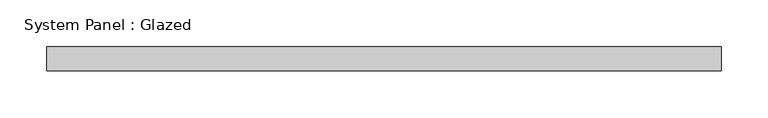
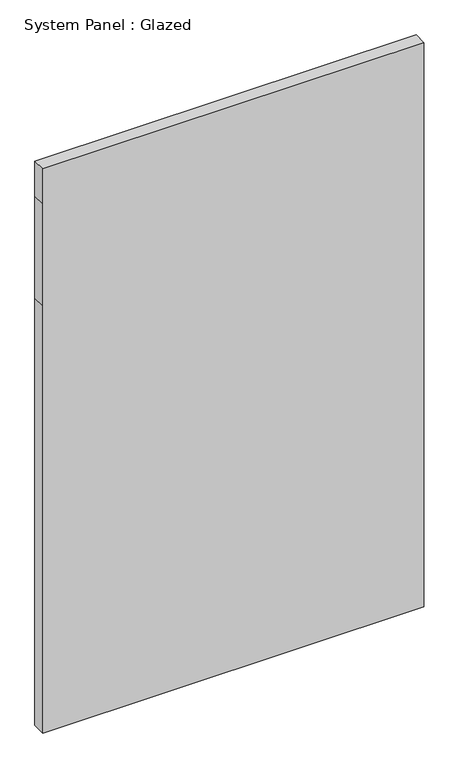
"""IFC4 building model written with IfcOpenShell, lengths in millimetres: plate geometry, System Panel : Glazed."""

from ifc_helpers import new_model, si_unit, frame, origin, place, context, project, spatial, polyline, outline, extrude, source, transform, mapped, element, save


def system_panel_glazed_66e670ab(model_context):
    return source(origin(), model_context, "Body", "SweptSolid", [
        extrude(outline(polyline([(0.0, -358.775), (0.0, 358.775), (850.299557, 358.775), (1053.3661252, 358.775), (1123.1494093, 358.775), (1123.1494093, -358.775), (1053.3661252, -358.775), (850.299557, -358.775), (0.0, -358.775)])), frame((0.0, 19.05, 0.0), z_axis=(0.0, 1.0, 0.0), x_axis=(0.0, 0.0, 1.0)), (0.0, 0.0, 1.0), 25.4),
    ])


if __name__ == "__main__":
    model = new_model("IFC4")
    model_context = context("Model", 3, world=origin())
    ifc_project = project(units=[si_unit("LENGTHUNIT", "METRE", prefix="MILLI")], contexts=[model_context])
    site = spatial("IfcSite", under=ifc_project)
    building = spatial("IfcBuilding", under=site)
    placement = place(None, origin())
    system_panel_glazed_shape = system_panel_glazed_66e670ab(model_context)
    element("IfcPlate", 1, ObjectType="System Panel : Glazed", at=placement, inside=building, context=model_context, shape_type="MappedRepresentation", body=[
        mapped(system_panel_glazed_shape, transform((0.0, 0.0, 0.0), x_axis=(1.0, 0.0, 0.0), y_axis=(0.0, 1.0, 0.0), z_axis=(0.0, 0.0, 1.0))),
    ])
    save(model, "model.ifc")

# Revit data of these elements
# Type "System Panel : Glazed"
#   Construction Type Id = "GSP4R"
#   Analytic Construction = "1/8 in Pilkington single glazing"
#   Visual Light Transmittance = 0.9
#   Solar Heat Gain Coefficient = 0.86
#   Heat Transfer Coefficient (U) = 1.18115 BTU/(h·ft²·°F)
#   Define Thermal Properties by = 1
# Element 1 (IfcPlate, "System Panel : Glazed")
#   Materials on its faces: "Glass"
# Materials
#   "Glass": class "Glass", colour RGB 0 128 192, transparency 0.75, Description = "Soda Lime Glass", Cost = 0
